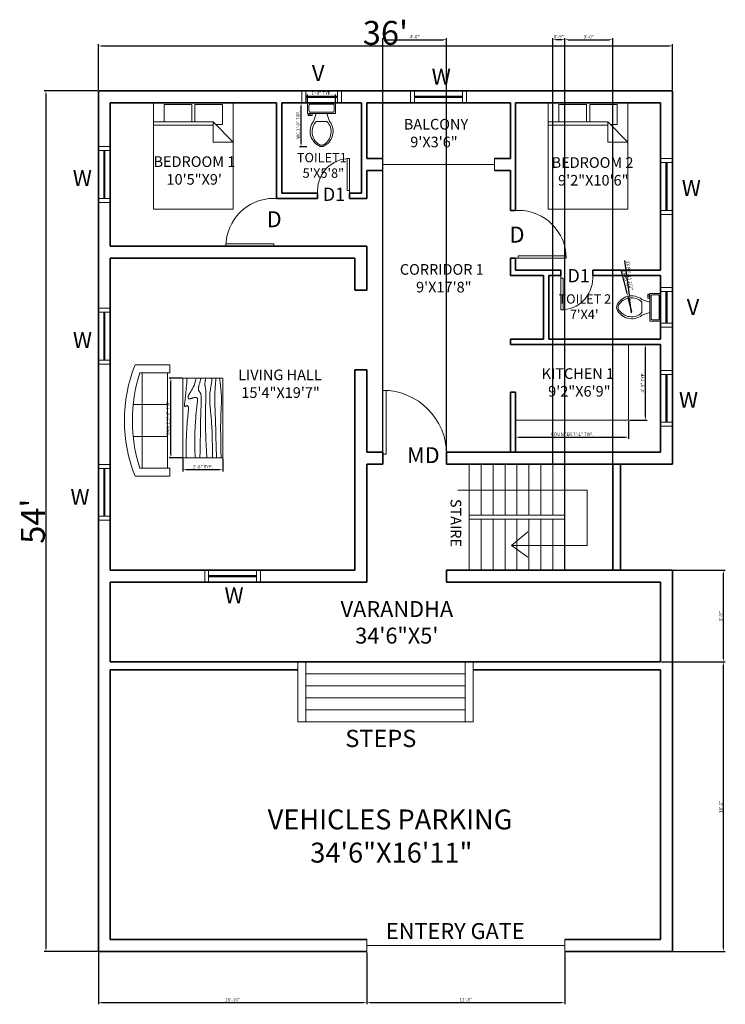
# Model space of a CAD drawing. Units: inches. Extents: x 2391 to 16591, y 7259 to 10239.
# Tile 27 of 27: x 16060 to 16591, y 9181 to 9922. Entities that reach past the tile are written whole.
import ezdxf

# ---------------------------------------------------------------- set-up
doc = ezdxf.new("R2010")
doc.units = ezdxf.units.IN
for name, color, linetype, lineweight in [('A-ANNO-DIMS', 4, 'Continuous', 18), ('A-ANNO-IDEN', 2, 'Continuous', 18), ('A-ANNO-SYMB', 3, 'Continuous', 18), ('A-AREA-IDEN', 7, 'Continuous', 18), ('A-DOOR', 3, 'Continuous', 18), ('A-FLOR-CASE', 6, 'Continuous', 18), ('A-FLOR-FIXT', 9, 'Continuous', 18), ('A-FLOR-HRAL', 8, 'Continuous', 18), ('A-FLOR-STRS', 7, 'Continuous', 18), ('A-FURN', 8, 'Continuous', 18), ('A-GLAZ', 4, 'Continuous', 18), ('A-WALL', 7, 'Continuous', 35)]:
    doc.layers.add(name, color=color, linetype=linetype, lineweight=lineweight)
doc.styles.get("Standard").update_dxf_attribs({"font": 'arial.ttf'})
doc.dimstyles.new('ISO-25', dxfattribs={"dimtxt": 2.5, "dimasz": 2.5, "dimexe": 1.25, "dimexo": 0.625, "dimtad": 1, "dimdec": 0, "dimlunit": 3, "dimtxsty": 'Standard', "dimcen": 2.5, "dimadec": 0, "dimazin": 0, "dimtfac": 1, "dimtdec": 0, "dimtmove": 0, "dimatfit": 3, "dimfxl": 1, "dimarcsym": 0})

# ---------------------------------------------------------------- blocks, each defined once
blk = doc.blocks.new('*U11')
for p, q in [((-36, 0), (-36, 6)), ((0, 0), (0, 6))]:
    blk.add_line(p, q)
blk.add_lwpolyline([(0, 0), (0, -36), (-1.75, -36), (-1.75, 0)], close=True)
blk.add_arc((0, 0), 36, 180, 270)
blk = doc.blocks.new('*U8')
for p, q in [((-24, 0), (-24, -6)), ((0, 0), (0, -6))]:
    blk.add_line(p, q)
blk.add_lwpolyline([(0, 0), (0, 24), (-1.75, 24), (-1.75, 0)], close=True)
blk.add_arc((0, 0), 24, 90, 180)
blk = doc.blocks.new('*U12')
for p, q in [((0, 0), (0, -6)), ((-36, 0), (-36, -6))]:
    blk.add_line(p, q)
blk.add_lwpolyline([(0, 0), (0, 36), (-1.75, 36), (-1.75, 0)], close=True)
blk.add_arc((0, 0), 36, 90, 180)
blk = doc.blocks.new('*U9')
for p, q in [((0, 0), (0, 6)), ((24, 0), (24, 6))]:
    blk.add_line(p, q)
blk.add_lwpolyline([(0, 0), (0, -24), (1.75, -24), (1.75, 0)], close=True)
blk.add_arc((0, 0), 24, 270, 0)
blk = doc.blocks.new('*U18')
for p, q in [((0, 0), (0, -5)), ((32, 0), (32, -5))]:
    blk.add_line(p, q)
blk.add_lwpolyline([(0, 0), (0, 32), (1.75, 32), (1.75, 0)], close=True)
blk.add_arc((0, 0), 32, 0, 90)
blk = doc.blocks.new('Bed - Queen')
for p, q in [((0, -80.00003), (0, 0)), ((0, 0), (59.99999, 0)), ((59.99999, 0), (59.99999, -80.00003)), ((7.99999, -1.2), (28.79998, -1.2)), ((7.99999, -14.4), (7.99999, -1.2)), ((28.79998, -1.2), (28.79998, -14.4)), ((31.19999, -1.2), (51.99999, -1.2)), ((31.19999, -14.4), (31.19999, -1.2)), ((51.99999, -1.2), (51.99999, -16.4)), ((0, -14.4), (44.8, -14.4)), ((59.99999, -29.6), (44.8, -14.4)), ((44.8, -14.4), (44.8, -29.6)), ((44.8, -16.8), (0, -16.8)), ((51.99999, -16.4), (46.79936, -16.4)), ((44.8, -29.6), (59.99999, -29.6)), ((59.99999, -80.00003), (0, -80.00003))]:
    blk.add_line(p, q)
blk = doc.blocks.new('Toilet - top')
for p, q in [((9.5, -6), (9.5, -2)), ((-10, -8.5), (-8, -8.5)), ((-10, -9.5), (-10, -8.5)), ((-7, -9.5), (-10, -9.5)), ((-8, -8.5), (-8, -8)), ((-7, -8), (-7, -9.5)), ((-4, -8), (-6, -14)), ((4, -14), (-4, -14)), ((4, -8), (6, -14))]:
    blk.add_line(p, q)
blk.add_lwpolyline([(10.5, -8), (10.5, 0), (-10.5, 0), (-10.5, -8)], close=True)
for points in [[(-9.5, -2), (-9.5, -6)], [(8.5, -1), (-8.5, -1)], [(-8.5, -7), (8.5, -7)]]:
    blk.add_lwpolyline(points)
for centre, radius, start, end in [((-8.62, -1.88), 0.884, 81.8699, 188.1301), ((-8.62, -6.12), 0.884, 171.8699, 278.1301), ((8.62, -1.88), 0.884, 351.8699, 98.1301), ((8.62, -6.12), 0.884, 261.8699, 8.1301), ((3.52, -21.58), 12.17, 141.46911, 247.97143), ((4.2, -21.82), 11.33, 136.36773, 238.94682), ((-3.52, -21.58), 12.17, 292.02843, 38.53071), ((-4.2, -21.82), 11.33, 301.05301, 43.63209), ((0, -27.88), 4, 245.73182, 294.26817), ((0, -29), 4, 254.86053, 285.13947)]:
    blk.add_arc(centre, radius, start, end)
blk = doc.blocks.new('Sofa - Roundback 7 ft.')
for p, q in [((-12.00002, -32.4421), (-12.00003, -6.5971)), ((11.99997, -32.4421), (11.99998, -6.5971)), ((-36.000027, -34), (-36.000027, -11.4696)), ((-35.999844, -13.3819), (35.9998, -13.3819)), ((35.99998, -34), (35.99998, -11.4696)), ((-36.000027, -32.4421), (35.99998, -32.4421))]:
    blk.add_line(p, q)
for points in [[(-36.000027, -34), (-42.000027, -34), (-42.000027, -8)], [(41.99998, -8), (41.99998, -34), (35.99998, -34)]]:
    blk.add_lwpolyline(points)
for centre, radius, start, end in [((0, -114.25), 114.25, 68.43141, 111.5686), ((-0.00001, -127.1968), 121.1968, 72.72033, 107.2797)]:
    blk.add_arc(centre, radius, start, end)
blk = doc.blocks.new('Table - Rectangular Woodgrain 60 x 30 in.')
for p, q in [((0, 0), (0, -30)), ((60, 0), (0, 0)), ((60, -30), (60, 0)), ((0, -30), (60, -30))]:
    blk.add_line(p, q)
for points in [[(0, -2.4), (4.8155, -2.418), (9.0302, -2.4688), (12.709, -2.5477), (15.9167, -2.65), (18.7181, -2.7711), (21.1781, -2.9063), (23.3616, -3.0508), (25.3333, -3.2), (27.1477, -3.3495), (28.8172, -3.4958), (30.3437, -3.636), (31.7291, -3.7667), (32.9756, -3.8849), (34.0849, -3.9875), (35.059, -4.0714), (35.9, -4.1334), (36.6114, -4.1711), (37.2041, -4.1854), (37.6906, -4.1779), (38.0833, -4.15), (38.3948, -4.1034), (38.6375, -4.0396), (38.8239, -3.9602), (38.9666, -3.8667), (39.0764, -3.7608), (39.1573, -3.6448), (39.2116, -3.521), (39.2416, -3.3917), (39.2498, -3.2593), (39.2385, -3.1261), (39.21, -2.9944), (39.1666, -2.8667), (39.111, -2.7447), (39.0468, -2.6281), (38.978, -2.5163), (38.9083, -2.4083), (38.8418, -2.3035), (38.7823, -2.201), (38.7337, -2.1001), (38.7, -2), (38.6844, -1.9003), (38.6875, -1.8021), (38.7094, -1.707), (38.75, -1.6167), (38.8094, -1.5326), (38.8875, -1.4563), (38.9844, -1.3893), (39.1, -1.3333), (39.2351, -1.2896), (39.3937, -1.2583), (39.5804, -1.2396), (39.8, -1.2333), (40.057, -1.2396), (40.3562, -1.2583), (40.7023, -1.2896), (41.1, -1.3333), (41.5547, -1.3895), (42.0755, -1.4573), (42.6721, -1.5361), (43.3542, -1.625), (44.1316, -1.7233), (45.014, -1.8302), (46.0114, -1.9449), (47.1333, -2.0667), (48.3862, -2.1947), (49.7625, -2.3281), (51.2513, -2.4663), (52.8416, -2.6083), (54.5226, -2.7535), (56.2833, -2.9011), (58.1127, -3.0501), (60, -3.2)], [(0, -9.2), (6.5759, -9.0858), (11.9385, -9.0365), (16.2527, -9.0418), (19.6833, -9.0917), (22.3952, -9.1759), (24.5531, -9.2844), (26.322, -9.4069), (27.8666, -9.5333), (29.3241, -9.6553), (30.7203, -9.7719), (32.0532, -9.8837), (33.3208, -9.9917), (34.5213, -10.0965), (35.6526, -10.199), (36.7128, -10.2999), (37.7, -10.4), (38.6129, -10.4996), (39.4531, -10.5969), (40.223, -10.6895), (40.925, -10.775), (41.5613, -10.8512), (42.1344, -10.9156), (42.6465, -10.966), (43.1, -11), (43.4976, -11.0158), (43.8437, -11.0136), (44.143, -10.9942), (44.4, -10.9583), (44.6195, -10.9069), (44.8062, -10.8406), (44.9648, -10.7603), (45.1, -10.6667), (45.2155, -10.5598), (45.3114, -10.4365), (45.3871, -10.2929), (45.4416, -10.125), (45.4743, -9.929), (45.4844, -9.7011), (45.4709, -9.4371), (45.4333, -9.1333), (45.3716, -8.7883), (45.2896, -8.4104), (45.1919, -8.0107), (45.0833, -7.6), (44.9685, -7.1893), (44.8521, -6.7896), (44.7388, -6.4117), (44.6333, -6.0667), (44.54, -5.7628), (44.4614, -5.4979), (44.4001, -5.2675), (44.3583, -5.0667), (44.3384, -4.8909), (44.3427, -4.7354), (44.3736, -4.5956), (44.4333, -4.4667), (44.5236, -4.3453), (44.6427, -4.2333), (44.7884, -4.1339), (44.9583, -4.05), (45.1501, -3.9849), (45.3614, -3.9417), (45.59, -3.9234), (45.8333, -3.9333), (46.0915, -3.9749), (46.3734, -4.0531), (46.6906, -4.1736), (47.0542, -4.3417), (47.4756, -4.5629), (47.9661, -4.8427), (48.5372, -5.1866), (49.2, -5.6), (49.9676, -6.0844), (50.8594, -6.625), (51.8965, -7.2031), (53.1, -7.8), (54.491, -8.3969), (56.0906, -8.975), (57.9199, -9.5156), (60, -10)], [(0, -12.8), (5.1847, -12.9322), (9.6213, -13.0323), (13.3963, -13.1059), (16.5958, -13.1583), (19.3063, -13.1952), (21.614, -13.2219), (23.6054, -13.2439), (25.3666, -13.2667), (26.9728, -13.2947), (28.4531, -13.3281), (29.8256, -13.3663), (31.1083, -13.4083), (32.3191, -13.4535), (33.476, -13.501), (34.597, -13.5501), (35.7, -13.6), (36.7984, -13.6497), (37.8875, -13.6979), (38.9578, -13.743), (40, -13.7833), (41.0047, -13.8174), (41.9625, -13.8438), (42.864, -13.8607), (43.7, -13.8667), (44.4631, -13.8604), (45.1552, -13.8417), (45.7801, -13.8104), (46.3416, -13.7667), (46.8439, -13.7104), (47.2906, -13.6417), (47.6858, -13.5604), (48.0333, -13.4667), (48.3375, -13.3608), (48.6042, -13.2448), (48.8396, -13.121), (49.05, -12.9917), (49.2417, -12.8593), (49.4208, -12.7261), (49.5937, -12.5944), (49.7667, -12.4667), (49.9452, -12.3451), (50.1323, -12.2313), (50.3303, -12.1268), (50.5416, -12.0333), (50.7686, -11.9524), (51.0135, -11.8854), (51.2788, -11.8341), (51.5666, -11.8), (51.8785, -11.7843), (52.2116, -11.7865), (52.562, -11.8059), (52.926, -11.8417), (53.2998, -11.8931), (53.6795, -11.9594), (54.0614, -12.0397), (54.4416, -12.1333), (54.8223, -12.2401), (55.2293, -12.3625), (55.6942, -12.5037), (56.2489, -12.6667), (56.9251, -12.8547), (57.7545, -13.0708), (58.7689, -13.3182), (60, -13.6)], [(0, -18), (5.124, -17.7273), (9.6609, -17.5057), (13.6705, -17.3303), (17.2125, -17.1958), (20.3467, -17.0973), (23.1328, -17.0297), (25.6307, -16.9878), (27.9, -16.9667), (29.9928, -16.9617), (31.9302, -16.9703), (33.7254, -16.9907), (35.3917, -17.0208), (36.9423, -17.0588), (38.3906, -17.1026), (39.7499, -17.1503), (41.0333, -17.2), (42.2519, -17.2496), (43.4073, -17.2969), (44.4986, -17.3395), (45.525, -17.375), (46.4858, -17.4012), (47.3802, -17.4156), (48.2074, -17.416), (48.9667, -17.4), (49.6583, -17.3662), (50.2872, -17.3167), (50.8595, -17.2547), (51.3812, -17.1833), (51.8584, -17.1057), (52.2971, -17.025), (52.7034, -16.9443), (53.0833, -16.8667), (53.443, -16.7951), (53.789, -16.7313), (54.128, -16.6768), (54.4666, -16.6334), (54.8115, -16.6024), (55.1693, -16.5854), (55.5465, -16.5841), (55.95, -16.6), (56.3828, -16.6337), (56.8346, -16.6823), (57.2915, -16.7418), (57.7396, -16.8084), (58.165, -16.878), (58.5539, -16.9469), (58.8924, -17.0111), (59.1666, -17.0667), (59.3679, -17.1107), (59.5078, -17.1438), (59.6032, -17.1675), (59.6708, -17.1833), (59.7275, -17.193), (59.7901, -17.1979), (59.8753, -17.1998), (60, -17.2)], [(0, -22.4), (8.0098, -22.2501), (14.4094, -22.1011), (19.4168, -21.9535), (23.25, -21.8083), (26.1269, -21.6663), (28.2656, -21.5281), (29.884, -21.3947), (31.2, -21.2667), (32.3967, -21.1448), (33.5172, -21.0292), (34.5697, -20.9198), (35.5625, -20.8167), (36.5037, -20.7198), (37.4015, -20.6292), (38.2642, -20.5448), (39.1, -20.4667), (39.9164, -20.3951), (40.7187, -20.3313), (41.5117, -20.2768), (42.3, -20.2333), (43.0883, -20.2024), (43.8812, -20.1854), (44.6836, -20.1841), (45.5, -20.2), (46.3328, -20.234), (47.1747, -20.2844), (48.0163, -20.3488), (48.8479, -20.425), (49.66, -20.5106), (50.4429, -20.6031), (51.1872, -20.7004), (51.8833, -20.8), (52.5246, -20.8999), (53.1166, -20.9995), (53.6681, -21.0983), (54.1875, -21.1958), (54.6834, -21.2919), (55.1646, -21.3859), (55.6394, -21.4777), (56.1167, -21.5667), (56.6028, -21.6515), (57.0961, -21.7266), (57.5929, -21.7852), (58.0896, -21.8208), (58.5823, -21.8268), (59.0674, -21.7964), (59.5412, -21.723), (60, -21.6)], [(0, -25.2), (8.6355, -25.0504), (15.7026, -24.9031), (21.4049, -24.7606), (25.9458, -24.625), (29.529, -24.4988), (32.3578, -24.3844), (34.6359, -24.284), (36.5667, -24.2), (38.3213, -24.1341), (39.9417, -24.0854), (41.437, -24.0523), (42.8167, -24.0333), (44.0901, -24.0268), (45.2667, -24.0313), (46.3557, -24.0451), (47.3667, -24.0667), (48.309, -24.0947), (49.1928, -24.1287), (50.0284, -24.168), (50.826, -24.2125), (51.5959, -24.2617), (52.3483, -24.3151), (53.0935, -24.3725), (53.8417, -24.4334), (54.6009, -24.497), (55.3699, -24.561), (56.1454, -24.6226), (56.9239, -24.6792), (57.7021, -24.7279), (58.4764, -24.7662), (59.2435, -24.7911), (60, -24.8)], [(0, -28.8), (5.6867, -28.6681), (10.45, -28.5698), (14.407, -28.5012), (17.675, -28.4584), (20.3711, -28.4374), (22.6125, -28.4344), (24.5164, -28.4455), (26.2, -28.4667), (27.762, -28.4947), (29.2276, -28.5281), (30.6033, -28.5663), (31.8958, -28.6084), (33.1118, -28.6535), (34.2578, -28.7011), (35.3405, -28.7501), (36.3666, -28.8), (37.3443, -28.8497), (38.288, -28.8974), (39.2137, -28.9412), (40.1375, -28.9792), (41.0753, -29.0093), (42.0432, -29.0297), (43.0572, -29.0384), (44.1333, -29.0333), (45.2936, -29.0114), (46.5843, -28.9641), (48.0579, -28.8816), (49.7666, -28.7542), (51.7629, -28.5721), (54.0989, -28.3255), (56.8272, -28.0048), (60, -27.6)]]:
    blk.add_lwpolyline(points)
blk = doc.blocks.new('*D25')
at = {"layer": 'A-ANNO-DIMS', "color": 0, "lineweight": -2, "transparency": 16777216}
for p, q in [((16119.06, 9868.94), (16119.06, 9903.36)), ((16121.56, 9902.11), (16548.56, 9902.11)), ((16551.06, 9868.94), (16551.06, 9903.36))]:
    blk.add_line(p, q, dxfattribs=at)
at = {"layer": 'A-ANNO-DIMS', "color": 0, "transparency": 16777216}
for points in [[(16121.56, 9902.52), (16121.56, 9901.69), (16119.06, 9902.11)], [(16548.56, 9902.52), (16548.56, 9901.69), (16551.06, 9902.11)]]:
    blk.add_solid(points, dxfattribs=at)
at = {"layer": 'Defpoints', "color": 0, "transparency": 16777216}
for p in [(16551.06, 9902.11), (16119.06, 9868.31), (16551.06, 9868.31)]:
    blk.add_point(p, dxfattribs=at)
at = {"layer": 'A-ANNO-DIMS', "color": 0, "transparency": 16777216, "insert": (16335.06, 9911.93), "char_height": 2.5, "attachment_point": 5}
blk.add_mtext("{\\H7.2x;36'}", dxfattribs=at)
blk = doc.blocks.new('*D26')
at = {"layer": 'A-ANNO-DIMS', "color": 0, "lineweight": -2, "transparency": 16777216}
for p, q in [((16118.43, 9868.31), (16078.34, 9868.31)), ((16079.59, 9865.81), (16079.59, 9222.81)), ((16118.43, 9220.31), (16078.34, 9220.31))]:
    blk.add_line(p, q, dxfattribs=at)
at = {"layer": 'A-ANNO-DIMS', "color": 0, "transparency": 16777216}
for points in [[(16079.18, 9865.81), (16080.01, 9865.81), (16079.59, 9868.31)], [(16079.18, 9222.81), (16080.01, 9222.81), (16079.59, 9220.31)]]:
    blk.add_solid(points, dxfattribs=at)
at = {"layer": 'Defpoints', "color": 0, "transparency": 16777216}
for p in [(16119.06, 9868.31), (16079.59, 9220.31), (16119.06, 9220.31)]:
    blk.add_point(p, dxfattribs=at)
at = {"layer": 'A-ANNO-DIMS', "color": 0, "transparency": 16777216, "insert": (16069.81, 9544.31), "char_height": 2.5, "attachment_point": 5, "rotation": 90}
blk.add_mtext("{\\H7.2x;54'}", dxfattribs=at)
blk = doc.blocks.new('WINDOW-36-PLAN')
for p, q in [((9, 42), (0, 42)), ((9, 39), (0, 39)), ((4, 39), (4, 3)), ((4.5, 39), (4.5, 3)), ((5, 39), (5, 3)), ((9, 3), (0, 3)), ((9, 0), (0, 0))]:
    blk.add_line(p, q)
blk = doc.blocks.new('VENT-24-PLAN')
for p, q in [((9, 30), (0, 30)), ((9, 27), (0, 27)), ((4, 27), (4, 3)), ((4.5, 27), (4.5, 3)), ((5, 27), (5, 3)), ((9, 3), (0, 3)), ((9, 0), (0, 0))]:
    blk.add_line(p, q)
blk = doc.blocks.new('STAIR-RETURN-FLIGHT')
for p, q in [((0, 80), (0, 0)), ((9, 80), (9, 41.5)), ((18, 80), (18, 41.5)), ((27, 80), (27, 41.5)), ((36, 80), (36, 41.5)), ((45, 80), (45, 41.5)), ((54, 80), (54, 41.5)), ((63, 80), (63, 41.5)), ((72, 80), (72, 0)), ((72, 41.5), (0, 41.5)), ((72, 38.5), (0, 38.5)), ((9, 38.5), (9, 0)), ((18, 38.5), (18, 0)), ((27, 38.5), (27, 0)), ((36, 38.5), (36, 0)), ((45, 38.5), (45, 0)), ((54, 38.5), (54, 0)), ((63, 38.5), (63, 0))]:
    blk.add_line(p, q)
blk = doc.blocks.new('STAIR-DIRECTION-ARROW')
for p, q in [((0, 50.31), (97.37, 50.31)), ((97.37, 50.31), (97.37, 8.81)), ((40.34, 8.81), (52.74, 18.89)), ((97.37, 8.81), (40.34, 8.81)), ((40.34, 8.81), (52.74, 0))]:
    blk.add_line(p, q)
blk = doc.blocks.new('COUNTER-L-KITCHEN-TYPE2')
for p in [(85, 57), (0, 0)]:
    blk.add_line(p, (85, 0))
blk = doc.blocks.new('STAIR-ENTRY-STEPS')
for p, q in [((0, 45), (0, 0)), ((6, 45), (6, 0)), ((126, 45), (126, 0)), ((132, 45), (132, 0)), ((6, 36), (126, 36)), ((6, 27), (126, 27)), ((6, 18), (126, 18)), ((6, 9), (126, 9)), ((0, 0), (132, 0))]:
    blk.add_line(p, q)
blk = doc.blocks.new('*D47')
at = {"layer": 'A-ANNO-DIMS', "color": 0, "lineweight": -2, "transparency": 16777216}
for p, q in [((16275.93, 9859.31), (16270.35, 9859.31)), ((16271.6, 9828.76), (16271.6, 9856.81)), ((16275.93, 9826.26), (16270.35, 9826.26))]:
    blk.add_line(p, q, dxfattribs=at)
at = {"layer": 'A-ANNO-DIMS', "color": 0, "transparency": 16777216}
for points in [[(16271.18, 9856.81), (16272.02, 9856.81), (16271.6, 9859.31)], [(16271.18, 9828.76), (16272.02, 9828.76), (16271.6, 9826.26)]]:
    blk.add_solid(points, dxfattribs=at)
at = {"layer": 'Defpoints', "color": 0, "transparency": 16777216}
for p in [(16271.6, 9859.31), (16276.56, 9859.31), (16276.56, 9826.26)]:
    blk.add_point(p, dxfattribs=at)
at = {"layer": 'A-ANNO-DIMS', "color": 0, "transparency": 16777216, "insert": (16269.68, 9842.79), "char_height": 2.5, "attachment_point": 5, "rotation": 90}
blk.add_mtext('WC 2\'-9" TYP.', dxfattribs=at)
blk = doc.blocks.new('*D48')
at = {"layer": 'A-ANNO-DIMS', "color": 0, "lineweight": -2, "transparency": 16777216}
for p, q in [((16276.56, 9859.94), (16276.56, 9865.52)), ((16279.06, 9864.27), (16295.06, 9864.27)), ((16297.56, 9859.94), (16297.56, 9865.52))]:
    blk.add_line(p, q, dxfattribs=at)
at = {"layer": 'A-ANNO-DIMS', "color": 0, "transparency": 16777216}
for points in [[(16279.06, 9864.68), (16279.06, 9863.85), (16276.56, 9864.27)], [(16295.06, 9864.68), (16295.06, 9863.85), (16297.56, 9864.27)]]:
    blk.add_solid(points, dxfattribs=at)
at = {"layer": 'Defpoints', "color": 0, "transparency": 16777216}
for p in [(16276.56, 9859.31), (16297.56, 9864.27), (16297.56, 9859.31)]:
    blk.add_point(p, dxfattribs=at)
at = {"layer": 'A-ANNO-DIMS', "color": 0, "transparency": 16777216, "insert": (16287.06, 9866.17), "char_height": 2.5, "attachment_point": 5}
blk.add_mtext('1\'-9" TYP.', dxfattribs=at)
blk = doc.blocks.new('*D51')
at = {"layer": 'A-ANNO-DIMS', "color": 0, "lineweight": -2, "transparency": 16777216}
for p, q in [((16182.02, 9652.03), (16172.39, 9652.03)), ((16173.64, 9594.53), (16173.64, 9649.53)), ((16182.02, 9592.03), (16172.39, 9592.03))]:
    blk.add_line(p, q, dxfattribs=at)
at = {"layer": 'A-ANNO-DIMS', "color": 0, "transparency": 16777216}
for points in [[(16173.23, 9649.53), (16174.06, 9649.53), (16173.64, 9652.03)], [(16173.23, 9594.53), (16174.06, 9594.53), (16173.64, 9592.03)]]:
    blk.add_solid(points, dxfattribs=at)
at = {"layer": 'Defpoints', "color": 0, "transparency": 16777216}
for p in [(16173.64, 9652.03), (16182.64, 9652.03), (16182.64, 9592.03)]:
    blk.add_point(p, dxfattribs=at)
at = {"layer": 'A-ANNO-DIMS', "color": 0, "transparency": 16777216, "insert": (16171.74, 9622.03), "char_height": 2.5, "attachment_point": 5, "rotation": 90}
blk.add_mtext('TABLE 5\'-0" TYP.', dxfattribs=at)
blk = doc.blocks.new('*D52')
at = {"layer": 'A-ANNO-DIMS', "color": 0, "lineweight": -2, "transparency": 16777216}
for p, q in [((16182.64, 9591.4), (16182.64, 9581.78)), ((16212.64, 9591.4), (16212.64, 9581.78)), ((16210.14, 9583.03), (16185.14, 9583.03))]:
    blk.add_line(p, q, dxfattribs=at)
at = {"layer": 'A-ANNO-DIMS', "color": 0, "transparency": 16777216}
for points in [[(16185.14, 9583.45), (16185.14, 9582.61), (16182.64, 9583.03)], [(16210.14, 9583.45), (16210.14, 9582.61), (16212.64, 9583.03)]]:
    blk.add_solid(points, dxfattribs=at)
at = {"layer": 'Defpoints', "color": 0, "transparency": 16777216}
for p in [(16182.64, 9592.03), (16212.64, 9592.03), (16182.64, 9583.03)]:
    blk.add_point(p, dxfattribs=at)
at = {"layer": 'A-ANNO-DIMS', "color": 0, "transparency": 16777216, "insert": (16197.64, 9584.93), "char_height": 2.5, "attachment_point": 5}
blk.add_mtext('2\'-6" TYP.', dxfattribs=at)
blk = doc.blocks.new('*D55')
at = {"layer": 'A-ANNO-DIMS', "color": 0, "lineweight": -2, "transparency": 16777216}
for p, q in [((16433.06, 9619.69), (16433.06, 9606.31)), ((16518.06, 9619.69), (16518.06, 9606.31)), ((16435.56, 9607.56), (16515.56, 9607.56))]:
    blk.add_line(p, q, dxfattribs=at)
at = {"layer": 'A-ANNO-DIMS', "color": 0, "transparency": 16777216}
for points in [[(16435.56, 9607.98), (16435.56, 9607.14), (16433.06, 9607.56)], [(16515.56, 9607.98), (16515.56, 9607.14), (16518.06, 9607.56)]]:
    blk.add_solid(points, dxfattribs=at)
at = {"layer": 'Defpoints', "color": 0, "transparency": 16777216}
for p in [(16433.06, 9620.31), (16518.06, 9620.31), (16518.06, 9607.56)]:
    blk.add_point(p, dxfattribs=at)
at = {"layer": 'A-ANNO-DIMS', "color": 0, "transparency": 16777216, "insert": (16475.56, 9609.48), "char_height": 2.5, "attachment_point": 5}
blk.add_mtext('COUNTER 7\'-1" TYP.', dxfattribs=at)
blk = doc.blocks.new('*D56')
at = {"layer": 'A-ANNO-DIMS', "color": 0, "lineweight": -2, "transparency": 16777216}
for p, q in [((16518.68, 9677.31), (16532.06, 9677.31)), ((16530.81, 9622.81), (16530.81, 9674.81)), ((16518.68, 9620.31), (16532.06, 9620.31))]:
    blk.add_line(p, q, dxfattribs=at)
at = {"layer": 'A-ANNO-DIMS', "color": 0, "transparency": 16777216}
for points in [[(16530.39, 9674.81), (16531.22, 9674.81), (16530.81, 9677.31)], [(16530.39, 9622.81), (16531.22, 9622.81), (16530.81, 9620.31)]]:
    blk.add_solid(points, dxfattribs=at)
at = {"layer": 'Defpoints', "color": 0, "transparency": 16777216}
for p in [(16518.06, 9677.31), (16530.81, 9677.31), (16518.06, 9620.31)]:
    blk.add_point(p, dxfattribs=at)
at = {"layer": 'A-ANNO-DIMS', "color": 0, "transparency": 16777216, "insert": (16528.91, 9648.81), "char_height": 2.5, "attachment_point": 5, "rotation": 90}
blk.add_mtext('4\'-9" TYP.', dxfattribs=at)
blk = doc.blocks.new('*D65')
at = {"layer": 'A-ANNO-DIMS', "color": 0, "lineweight": -2, "transparency": 16777216}
for p, q in [((16119.06, 9219.69), (16119.06, 9180.56)), ((16321.06, 9219.69), (16321.06, 9180.56)), ((16121.56, 9181.81), (16318.56, 9181.81))]:
    blk.add_line(p, q, dxfattribs=at)
at = {"layer": 'A-ANNO-DIMS', "color": 0, "transparency": 16777216}
for points in [[(16121.56, 9182.23), (16121.56, 9181.39), (16119.06, 9181.81)], [(16318.56, 9182.23), (16318.56, 9181.39), (16321.06, 9181.81)]]:
    blk.add_solid(points, dxfattribs=at)
at = {"layer": 'Defpoints', "color": 0, "transparency": 16777216}
for p in [(16119.06, 9220.31), (16321.06, 9220.31), (16321.06, 9181.81)]:
    blk.add_point(p, dxfattribs=at)
at = {"layer": 'A-ANNO-DIMS', "color": 0, "transparency": 16777216, "insert": (16220.06, 9183.71), "char_height": 2.5, "attachment_point": 5}
blk.add_mtext('16\'-10"', dxfattribs=at)
blk = doc.blocks.new('*D66')
at = {"layer": 'A-ANNO-DIMS', "color": 0, "lineweight": -2, "transparency": 16777216}
for p, q in [((16321.06, 9219.69), (16321.06, 9180.56)), ((16470.06, 9219.69), (16470.06, 9180.56)), ((16323.56, 9181.81), (16467.56, 9181.81))]:
    blk.add_line(p, q, dxfattribs=at)
at = {"layer": 'A-ANNO-DIMS', "color": 0, "transparency": 16777216}
for points in [[(16323.56, 9182.23), (16323.56, 9181.39), (16321.06, 9181.81)], [(16467.56, 9182.23), (16467.56, 9181.39), (16470.06, 9181.81)]]:
    blk.add_solid(points, dxfattribs=at)
at = {"layer": 'Defpoints', "color": 0, "transparency": 16777216}
for p in [(16321.06, 9220.31), (16470.06, 9220.31), (16470.06, 9181.81)]:
    blk.add_point(p, dxfattribs=at)
at = {"layer": 'A-ANNO-DIMS', "color": 0, "transparency": 16777216, "insert": (16395.56, 9183.71), "char_height": 2.5, "attachment_point": 5}
blk.add_mtext('12\'-5"', dxfattribs=at)
blk = doc.blocks.new('*D67')
at = {"layer": 'A-ANNO-DIMS', "color": 0, "lineweight": -2, "transparency": 16777216}
for p, q in [((16333.06, 9596.94), (16333.06, 9908.06)), ((16335.56, 9906.81), (16378.56, 9906.81)), ((16381.06, 9596.94), (16381.06, 9908.06))]:
    blk.add_line(p, q, dxfattribs=at)
at = {"layer": 'A-ANNO-DIMS', "color": 0, "transparency": 16777216}
for points in [[(16335.56, 9907.23), (16335.56, 9906.39), (16333.06, 9906.81)], [(16378.56, 9907.23), (16378.56, 9906.39), (16381.06, 9906.81)]]:
    blk.add_solid(points, dxfattribs=at)
at = {"layer": 'Defpoints', "color": 0, "transparency": 16777216}
for p in [(16381.06, 9906.81), (16333.06, 9596.31), (16381.06, 9596.31)]:
    blk.add_point(p, dxfattribs=at)
at = {"layer": 'A-ANNO-DIMS', "color": 0, "transparency": 16777216, "insert": (16357.06, 9908.71), "char_height": 2.5, "attachment_point": 5}
blk.add_mtext('4\'-0"', dxfattribs=at)
blk = doc.blocks.new('*D68')
at = {"layer": 'A-ANNO-DIMS', "color": 0, "lineweight": -2, "transparency": 16777216}
for p, q in [((16470.06, 9507.94), (16470.06, 9908.06)), ((16472.56, 9906.81), (16503.56, 9906.81)), ((16506.06, 9507.94), (16506.06, 9908.06))]:
    blk.add_line(p, q, dxfattribs=at)
at = {"layer": 'A-ANNO-DIMS', "color": 0, "transparency": 16777216}
for points in [[(16472.56, 9907.23), (16472.56, 9906.39), (16470.06, 9906.81)], [(16503.56, 9907.23), (16503.56, 9906.39), (16506.06, 9906.81)]]:
    blk.add_solid(points, dxfattribs=at)
at = {"layer": 'Defpoints', "color": 0, "transparency": 16777216}
for p in [(16506.06, 9906.81), (16470.06, 9507.31), (16506.06, 9507.31)]:
    blk.add_point(p, dxfattribs=at)
at = {"layer": 'A-ANNO-DIMS', "color": 0, "transparency": 16777216, "insert": (16488.06, 9908.71), "char_height": 2.5, "attachment_point": 5}
blk.add_mtext('3\'-0"', dxfattribs=at)
blk = doc.blocks.new('*D69')
at = {"layer": 'A-ANNO-DIMS', "color": 0, "lineweight": -2, "transparency": 16777216}
for p, q in [((16461.06, 9587.94), (16461.06, 9908.06)), ((16467.56, 9906.81), (16463.56, 9906.81)), ((16470.06, 9587.94), (16470.06, 9908.06))]:
    blk.add_line(p, q, dxfattribs=at)
at = {"layer": 'A-ANNO-DIMS', "color": 0, "transparency": 16777216}
for points in [[(16463.56, 9907.23), (16463.56, 9906.39), (16461.06, 9906.81)], [(16467.56, 9907.23), (16467.56, 9906.39), (16470.06, 9906.81)]]:
    blk.add_solid(points, dxfattribs=at)
at = {"layer": 'Defpoints', "color": 0, "transparency": 16777216}
for p in [(16461.06, 9906.81), (16461.06, 9587.31), (16470.06, 9587.31)]:
    blk.add_point(p, dxfattribs=at)
at = {"layer": 'A-ANNO-DIMS', "color": 0, "transparency": 16777216, "insert": (16465.56, 9908.71), "char_height": 2.5, "attachment_point": 5}
blk.add_mtext('0\'-9"', dxfattribs=at)
blk = doc.blocks.new('*D70')
at = {"layer": 'A-ANNO-DIMS', "color": 0, "lineweight": -2, "transparency": 16777216}
for p, q in [((16542.68, 9438.31), (16590.81, 9438.31)), ((16589.56, 9222.81), (16589.56, 9435.81)), ((16551.68, 9220.31), (16590.81, 9220.31))]:
    blk.add_line(p, q, dxfattribs=at)
at = {"layer": 'A-ANNO-DIMS', "color": 0, "transparency": 16777216}
for points in [[(16589.14, 9435.81), (16589.97, 9435.81), (16589.56, 9438.31)], [(16589.14, 9222.81), (16589.97, 9222.81), (16589.56, 9220.31)]]:
    blk.add_solid(points, dxfattribs=at)
at = {"layer": 'Defpoints', "color": 0, "transparency": 16777216}
for p in [(16542.06, 9438.31), (16589.56, 9438.31), (16551.06, 9220.31)]:
    blk.add_point(p, dxfattribs=at)
at = {"layer": 'A-ANNO-DIMS', "color": 0, "transparency": 16777216, "insert": (16587.66, 9329.31), "char_height": 2.5, "attachment_point": 5, "rotation": 90}
blk.add_mtext('18\'-2"', dxfattribs=at)
blk = doc.blocks.new('*D71')
at = {"layer": 'A-ANNO-DIMS', "color": 0, "lineweight": -2, "transparency": 16777216}
for p, q in [((16551.68, 9507.31), (16590.81, 9507.31)), ((16589.56, 9440.81), (16589.56, 9504.81)), ((16542.68, 9438.31), (16590.81, 9438.31))]:
    blk.add_line(p, q, dxfattribs=at)
at = {"layer": 'A-ANNO-DIMS', "color": 0, "transparency": 16777216}
for points in [[(16589.14, 9504.81), (16589.97, 9504.81), (16589.56, 9507.31)], [(16589.14, 9440.81), (16589.97, 9440.81), (16589.56, 9438.31)]]:
    blk.add_solid(points, dxfattribs=at)
at = {"layer": 'Defpoints', "color": 0, "transparency": 16777216}
for p in [(16551.06, 9507.31), (16589.56, 9507.31), (16542.06, 9438.31)]:
    blk.add_point(p, dxfattribs=at)
at = {"layer": 'A-ANNO-DIMS', "color": 0, "transparency": 16777216, "insert": (16587.66, 9472.81), "char_height": 2.5, "attachment_point": 5, "rotation": 90}
blk.add_mtext('5\'-9"', dxfattribs=at)
blk = doc.blocks.new('*D119')
at = {"layer": 'A-ANNO-DIMS', "color": 0, "lineweight": -2, "transparency": 16777216}
for p, q in [((16512.12, 9733.58), (16516.75, 9715.98)), ((16520.48, 9701.79), (16517.38, 9713.56))]:
    blk.add_line(p, q, dxfattribs=at)
at = {"layer": 'A-ANNO-DIMS', "color": 0, "transparency": 16777216}
blk.add_solid([(16517.15, 9716.08), (16516.35, 9715.87), (16517.38, 9713.56)], dxfattribs=at)
at = {"layer": 'Defpoints', "color": 0, "transparency": 16777216}
for p in [(16517.38, 9713.56), (16520.48, 9701.79)]:
    blk.add_point(p, dxfattribs=at)
at = {"layer": 'A-ANNO-DIMS', "color": 0, "transparency": 16777216, "insert": (16515.96, 9726.47), "char_height": 2.5, "attachment_point": 5, "rotation": 284.72184}
blk.add_mtext('2X R1\'-0"', dxfattribs=at)
blk = doc.blocks.new('*D120')
at = {"layer": 'A-ANNO-DIMS', "color": 0, "lineweight": -2, "transparency": 16777216}
for p, q in [((16514.94, 9740.56), (16518.4, 9714.82)), ((16520.24, 9701.11), (16518.73, 9712.34))]:
    blk.add_line(p, q, dxfattribs=at)
at = {"layer": 'A-ANNO-DIMS', "color": 0, "transparency": 16777216}
blk.add_solid([(16518.81, 9714.87), (16517.99, 9714.76), (16518.73, 9712.34)], dxfattribs=at)
at = {"layer": 'Defpoints', "color": 0, "transparency": 16777216}
for p in [(16518.73, 9712.34), (16520.24, 9701.11)]:
    blk.add_point(p, dxfattribs=at)
at = {"layer": 'A-ANNO-DIMS', "color": 0, "transparency": 16777216, "insert": (16518.4, 9729.18), "char_height": 2.5, "attachment_point": 5, "rotation": 277.6564}
blk.add_mtext('2X R0\'-11 1/2"', dxfattribs=at)

msp = doc.modelspace()

# ---------------------------------------------------------------- linework, layer by layer
at = {"layer": 'A-DOOR'}
for p, q in [((16321.06, 9229.31), (16321.06, 9220.31)), ((16470.06, 9229.31), (16470.06, 9220.31)), ((16321.06, 9224.81), (16470.06, 9224.81))]:
    msp.add_line(p, q, dxfattribs=at)
at = {"layer": 'A-FLOR-HRAL'}
for p, q in [((16333.06, 9808.31), (16333.06, 9817.31)), ((16417.06, 9808.31), (16417.06, 9817.31)), ((16333.06, 9812.81), (16417.06, 9812.81))]:
    msp.add_line(p, q, dxfattribs=at)
at = {"layer": 'A-WALL'}
for p, q in [((16119.06, 9868.31), (16551.06, 9868.31)), ((16119.06, 9220.31), (16119.06, 9868.31)), ((16551.06, 9868.31), (16551.06, 9587.31)), ((16128.06, 9859.31), (16253.06, 9859.31)), ((16128.06, 9751.31), (16128.06, 9859.31)), ((16253.06, 9787.31), (16253.06, 9859.31)), ((16257.06, 9859.31), (16317.06, 9859.31)), ((16257.06, 9791.31), (16257.06, 9859.31)), ((16317.06, 9791.31), (16317.06, 9859.31)), ((16321.06, 9859.31), (16429.06, 9859.31)), ((16321.06, 9817.31), (16321.06, 9859.31)), ((16429.06, 9817.31), (16429.06, 9859.31)), ((16433.06, 9859.31), (16542.06, 9859.31)), ((16433.06, 9778.31), (16433.06, 9859.31)), ((16542.06, 9859.31), (16542.06, 9733.31)), ((16321.06, 9817.31), (16333.06, 9817.31)), ((16417.06, 9817.31), (16429.06, 9817.31)), ((16321.06, 9808.31), (16333.06, 9808.31)), ((16321.06, 9787.31), (16321.06, 9808.31)), ((16417.06, 9808.31), (16429.06, 9808.31)), ((16429.06, 9778.31), (16429.06, 9808.31)), ((16253.06, 9787.31), (16284.06, 9787.31)), ((16257.06, 9791.31), (16284.06, 9791.31)), ((16284.06, 9787.31), (16284.06, 9791.31)), ((16308.06, 9791.31), (16317.06, 9791.31)), ((16308.06, 9787.31), (16308.06, 9791.31)), ((16308.06, 9787.31), (16321.06, 9787.31)), ((16429.06, 9778.31), (16433.06, 9778.31)), ((16128.06, 9751.31), (16321.06, 9751.31)), ((16321.06, 9718.31), (16321.06, 9751.31)), ((16128.06, 9742.31), (16312.06, 9742.31)), ((16128.06, 9507.31), (16128.06, 9742.31)), ((16312.06, 9718.31), (16312.06, 9742.31)), ((16429.06, 9742.31), (16433.06, 9742.31)), ((16429.06, 9729.31), (16429.06, 9742.31)), ((16433.06, 9733.31), (16433.06, 9742.31)), ((16433.06, 9733.31), (16467.06, 9733.31)), ((16467.06, 9733.31), (16467.06, 9729.31)), ((16491.06, 9733.31), (16542.06, 9733.31)), ((16491.06, 9733.31), (16491.06, 9729.31)), ((16429.06, 9729.31), (16454.06, 9729.31)), ((16454.06, 9729.31), (16454.06, 9681.31)), ((16458.06, 9729.31), (16467.06, 9729.31)), ((16458.06, 9729.31), (16458.06, 9681.31)), ((16491.06, 9729.31), (16542.06, 9729.31)), ((16542.06, 9729.31), (16542.06, 9681.31)), ((16312.06, 9718.31), (16321.06, 9718.31)), ((16429.06, 9681.31), (16454.06, 9681.31)), ((16429.06, 9677.31), (16429.06, 9681.31)), ((16429.06, 9677.31), (16542.06, 9677.31)), ((16458.06, 9681.31), (16542.06, 9681.31)), ((16542.06, 9677.31), (16542.06, 9596.31)), ((16312.06, 9658.31), (16321.06, 9658.31)), ((16312.06, 9507.31), (16312.06, 9658.31)), ((16321.06, 9596.31), (16321.06, 9658.31)), ((16429.06, 9641.31), (16433.06, 9641.31)), ((16429.06, 9596.31), (16429.06, 9641.31)), ((16433.06, 9596.31), (16433.06, 9641.31)), ((16321.06, 9596.31), (16333.06, 9596.31)), ((16333.06, 9587.31), (16333.06, 9596.31)), ((16381.06, 9596.31), (16542.06, 9596.31)), ((16381.06, 9587.31), (16381.06, 9596.31)), ((16321.06, 9587.31), (16333.06, 9587.31)), ((16321.06, 9498.31), (16321.06, 9587.31)), ((16381.06, 9587.31), (16551.06, 9587.31)), ((16506.06, 9587.31), (16506.06, 9507.31)), ((16512.06, 9587.31), (16512.06, 9507.31)), ((16128.06, 9507.31), (16312.06, 9507.31)), ((16381.06, 9507.31), (16551.06, 9507.31)), ((16381.06, 9498.31), (16381.06, 9507.31)), ((16551.06, 9507.31), (16551.06, 9220.31)), ((16128.06, 9498.31), (16321.06, 9498.31)), ((16128.06, 9438.31), (16128.06, 9498.31)), ((16381.06, 9498.31), (16542.06, 9498.31)), ((16542.06, 9498.31), (16542.06, 9438.31)), ((16128.06, 9438.31), (16321.06, 9438.31)), ((16128.06, 9438.31), (16542.06, 9438.31)), ((16128.06, 9432.31), (16269.06, 9432.31)), ((16128.06, 9229.31), (16128.06, 9432.31)), ((16401.06, 9432.31), (16542.06, 9432.31)), ((16542.06, 9432.31), (16542.06, 9229.31)), ((16321.06, 9229.31), (16128.06, 9229.31)), ((16542.06, 9229.31), (16470.06, 9229.31)), ((16321.06, 9220.31), (16119.06, 9220.31)), ((16551.06, 9220.31), (16470.06, 9220.31))]:
    msp.add_line(p, q, dxfattribs=at)

# ---------------------------------------------------------------- block references
at = {"layer": 'A-ANNO-SYMB'}
msp.add_blockref('STAIR-DIRECTION-ARROW', (16389.49, 9517.28), dxfattribs=at)
at = {"layer": 'A-DOOR'}
for name, p in [('*U8', (16308.06, 9793.31)), ('*U9', (16467.06, 9727.31))]:
    msp.add_blockref(name, p, dxfattribs=at)
at = {"layer": 'A-DOOR', "rotation": 270}
for name, p in [('*U11', (16251.06, 9751.31)), ('*U12', (16435.06, 9742.31))]:
    msp.add_blockref(name, p, dxfattribs=at)
at = {"layer": 'A-DOOR', "xscale": 1.5, "yscale": 1.5, "zscale": 1.5}
msp.add_blockref('*U18', (16333.06, 9594.81), dxfattribs=at)
at = {"layer": 'A-FLOR-CASE'}
msp.add_blockref('COUNTER-L-KITCHEN-TYPE2', (16433.06, 9620.31), dxfattribs=at)
at = {"layer": 'A-FLOR-FIXT'}
msp.add_blockref('Toilet - top', (16287.06, 9859.31), dxfattribs=at)
at = {"layer": 'A-FLOR-FIXT', "rotation": 270}
msp.add_blockref('Toilet - top', (16542.06, 9705.31), dxfattribs=at)
at = {"layer": 'A-FLOR-STRS', "rotation": 180}
msp.add_blockref('STAIR-RETURN-FLIGHT', (16470.06, 9587.31), dxfattribs=at)
at = {"layer": 'A-FLOR-STRS'}
msp.add_blockref('STAIR-ENTRY-STEPS', (16269.06, 9393.31), dxfattribs=at)
at = {"layer": 'A-FURN'}
for p in [(16160.56, 9859.31), (16457.56, 9859.31)]:
    msp.add_blockref('Bed - Queen', p, dxfattribs=at)
at = {"layer": 'A-FURN', "rotation": 90}
for name, p in [('Sofa - Roundback 7 ft.', (16138.73, 9620.09)), ('Table - Rectangular Woodgrain 60 x 30 in.', (16182.64, 9592.03))]:
    msp.add_blockref(name, p, dxfattribs=at)
at = {"layer": 'A-GLAZ'}
for name, p, rotation in [('VENT-24-PLAN', (16302.06, 9859.31), 89.99999999999613), ('WINDOW-36-PLAN', (16396.06, 9859.31), 90.00000000000205), ('WINDOW-36-PLAN', (16128.06, 9826.31), 180), ('WINDOW-36-PLAN', (16551.06, 9817.31), 180), ('VENT-24-PLAN', (16551.06, 9720.31), 180), ('WINDOW-36-PLAN', (16128.06, 9704.56), 180), ('WINDOW-36-PLAN', (16551.06, 9657.81), 180), ('WINDOW-36-PLAN', (16128.06, 9587.06), 180), ('WINDOW-36-PLAN', (16241.06, 9498.31), 90.00000000000676)]:
    msp.add_blockref(name, p, dxfattribs=dict(at, rotation=rotation))

# ---------------------------------------------------------------- texts
at = {"layer": 'A-ANNO-IDEN', "attachment_point": 1}
for s, width, insert, char_height in [('V', 17.0712, (16279.75, 9887.64), 12), ('W', 41.0391, (16369.88, 9884.88), 12), ('W', 41.0391, (16099.82, 9808.62), 12), ('W', 41.0391, (16558.05, 9801.21), 12), ('D1', 88.0557, (16287.92, 9795.43), 10), ('D', 711.4851, (16245.73, 9777.62), 12), ('D', 711.4851, (16428.47, 9766.05), 12), ('D1', 88.0557, (16472, 9734.12), 10), ('V', 17.0712, (16561.81, 9711.52), 12), ('W', 41.0391, (16099.91, 9686.71), 12), ('W', 41.0391, (16555.93, 9641.66), 12), ('MD', 711.4851, (16351.3, 9600), 12), ('W', 41.0391, (16098.07, 9568.61), 12), ('W', 41.0391, (16213.97, 9494.56), 12)]:
    msp.add_mtext_dynamic_manual_height_columns(s, width=width, gutter_width=12.5, heights=[0], dxfattribs=dict(at, insert=insert, char_height=char_height))
at = {"layer": 'A-AREA-IDEN', "attachment_point": 1}
for s, width, insert, char_height in [('BALCONY\\P  9\'X3\'6"', 125.309, (16348.87, 9847.14), 8), ('BEDROOM 1\\P    10\'5"X9\'', 152.4027, (16160.56, 9818.98), 8), ('TOILET1\\P  5\'X5\'8"', 175.2431, (16268.49, 9821.54), 7), ('BEDROOM 2\\P  9\'2"X10\'6"', 186.7643, (16460.12, 9818.3), 8), ('CORRIDOR 1\\P     9\'X17\'8"', 386.0733, (16345.91, 9737.84), 8), ("{\\H0.875x;TOILET 2\\P    7'X4}'", 130.8261, (16465.34, 9715.11), 8), ('KITCHEN 1\\P  9\'2"X6\'9"', 260.4884, (16452.66, 9659.42), 8), ('LIVING HALL\\P 15\'4"X19\'7"', 316.1653, (16224.23, 9658.46), 8), ('VARANDHA\\P   34\'6"X5\'', 463.6702, (16301.33, 9484.14), 12), ('{STEPS}', 155.1331, (16304.87, 9387.23), 13), ('VEHICLES PARKING\\P       34\'6"X16\'11"', 315.868, (16246.45, 9327.25), 15), ('ENTERY GATE', 133.1329, (16335.46, 9241.71), 12)]:
    msp.add_mtext_dynamic_manual_height_columns(s, width=width, gutter_width=12.5, heights=[0], dxfattribs=dict(at, insert=insert, char_height=char_height))
at = {"layer": 'A-AREA-IDEN', "insert": (16392.11, 9561.07), "char_height": 8, "attachment_point": 1, "rotation": 270}
msp.add_mtext_dynamic_manual_height_columns('STAIRE', width=212.5876, gutter_width=12.5, heights=[0], dxfattribs=at)

# ---------------------------------------------------------------- dimensions: what is measured, and where the dimension line sits
at = {"layer": 'A-ANNO-DIMS'}
for base, p1, p2, text, override, picture, middle in [((16551.06, 9902.11), (16119.06, 9868.31), (16551.06, 9868.31), '{\\H7.2x;<>}', {"dimclrd": 0, "dimclre": 0, "dimclrt": 0}, '*D25', (16335.06, 9911.93)), ((16297.56, 9864.27), (16276.56, 9859.31), (16297.56, 9859.31), '<> TYP.', {"dimdec": 1, "dimlfac": 1, "dimrnd": 0, "dimzin": 1, "dimdsep": 46, "dimlunit": 4, "dimfrac": 2}, '*D48', (16287.06, 9866.17)), ((16518.06, 9607.56), (16433.06, 9620.31), (16518.06, 9620.31), 'COUNTER <> TYP.', {"dimdec": 1, "dimlfac": 1, "dimrnd": 0, "dimzin": 1, "dimdsep": 46, "dimlunit": 4, "dimfrac": 2}, '*D55', (16475.56, 9609.48))]:
    dim = msp.add_linear_dim(base=base, p1=p1, p2=p2, text=text, dimstyle='ISO-25', override=override, dxfattribs=at)
    dim.commit()
    dim.dimension.update_dxf_attribs({"geometry": picture, "text_midpoint": middle})
for base, p1, p2, picture, middle in [((16381.06, 9906.81), (16333.06, 9596.31), (16381.06, 9596.31), '*D67', (16357.06, 9908.71)), ((16461.06, 9906.81), (16470.06, 9587.31), (16461.06, 9587.31), '*D69', (16465.56, 9908.71)), ((16506.06, 9906.81), (16470.06, 9507.31), (16506.06, 9507.31), '*D68', (16488.06, 9908.71)), ((16321.06, 9181.81), (16119.06, 9220.31), (16321.06, 9220.31), '*D65', (16220.06, 9183.71)), ((16470.06, 9181.81), (16321.06, 9220.31), (16470.06, 9220.31), '*D66', (16395.56, 9183.71))]:
    dim = msp.add_linear_dim(base=base, p1=p1, p2=p2, dimstyle='ISO-25', override={"dimdec": 1, "dimlfac": 1, "dimrnd": 0, "dimzin": 1, "dimdsep": 46, "dimlunit": 4, "dimfrac": 2}, dxfattribs=at)
    dim.commit()
    dim.dimension.update_dxf_attribs({"geometry": picture, "text_midpoint": middle})
for base, p1, p2, angle, text, override, picture, middle in [((16079.59, 9220.31), (16119.06, 9868.31), (16119.06, 9220.31), 90, '{\\H7.2x;<>}', {"dimclrd": 0, "dimclre": 0, "dimclrt": 0}, '*D26', (16069.81, 9544.31)), ((16271.6009, 9859.3104), (16276.5579, 9826.2642), (16276.5579, 9859.3104), 90, 'WC <> TYP.', {"dimdec": 1, "dimlfac": 1, "dimrnd": 0, "dimzin": 1, "dimdsep": 46, "dimlunit": 4, "dimfrac": 2}, '*D47', (16269.6833, 9842.7873)), ((16530.81, 9677.31), (16518.06, 9620.31), (16518.06, 9677.31), 90, '<> TYP.', {"dimdec": 1, "dimlfac": 1, "dimrnd": 0, "dimzin": 1, "dimdsep": 46, "dimlunit": 4, "dimfrac": 2}, '*D56', (16528.91, 9648.81)), ((16173.64, 9652.03), (16182.64, 9592.03), (16182.64, 9652.03), 90, 'TABLE <> TYP.', {"dimdec": 1, "dimlfac": 1, "dimrnd": 0, "dimzin": 1, "dimdsep": 46, "dimlunit": 4, "dimfrac": 2}, '*D51', (16171.74, 9622.03)), ((16182.64, 9583.03), (16212.64, 9592.03), (16182.64, 9592.03), 180, '<> TYP.', {"dimdec": 1, "dimlfac": 1, "dimrnd": 0, "dimzin": 1, "dimdsep": 46, "dimlunit": 4, "dimfrac": 2}, '*D52', (16197.64, 9584.93))]:
    dim = msp.add_linear_dim(base=base, p1=p1, p2=p2, angle=angle, text=text, dimstyle='ISO-25', override=override, dxfattribs=at)
    dim.commit()
    dim.dimension.update_dxf_attribs({"geometry": picture, "text_midpoint": middle})
for center, mpoint, picture, middle in [((16520.48, 9701.79), (16517.38, 9713.56), '*D119', (16515.96, 9726.47)), ((16520.24, 9701.11), (16518.73, 9712.34), '*D120', (16518.4, 9729.18))]:
    dim = msp.add_radius_dim(center=center, mpoint=mpoint, text='2X <>', dimstyle='ISO-25', override={"dimdec": 1, "dimlfac": 1, "dimrnd": 0, "dimzin": 1, "dimdsep": 46, "dimlunit": 4, "dimfrac": 2}, dxfattribs=at)
    dim.commit()
    dim.dimension.update_dxf_attribs({"geometry": picture, "text_midpoint": middle})
for base, p1, p2, picture, middle in [((16589.56, 9507.31), (16542.06, 9438.31), (16551.06, 9507.31), '*D71', (16587.66, 9472.81)), ((16589.56, 9438.31), (16551.06, 9220.31), (16542.06, 9438.31), '*D70', (16587.66, 9329.31))]:
    dim = msp.add_linear_dim(base=base, p1=p1, p2=p2, angle=90, dimstyle='ISO-25', override={"dimdec": 1, "dimlfac": 1, "dimrnd": 0, "dimzin": 1, "dimdsep": 46, "dimlunit": 4, "dimfrac": 2}, dxfattribs=at)
    dim.commit()
    dim.dimension.update_dxf_attribs({"geometry": picture, "text_midpoint": middle})

doc.saveas('drawing.dxf')
